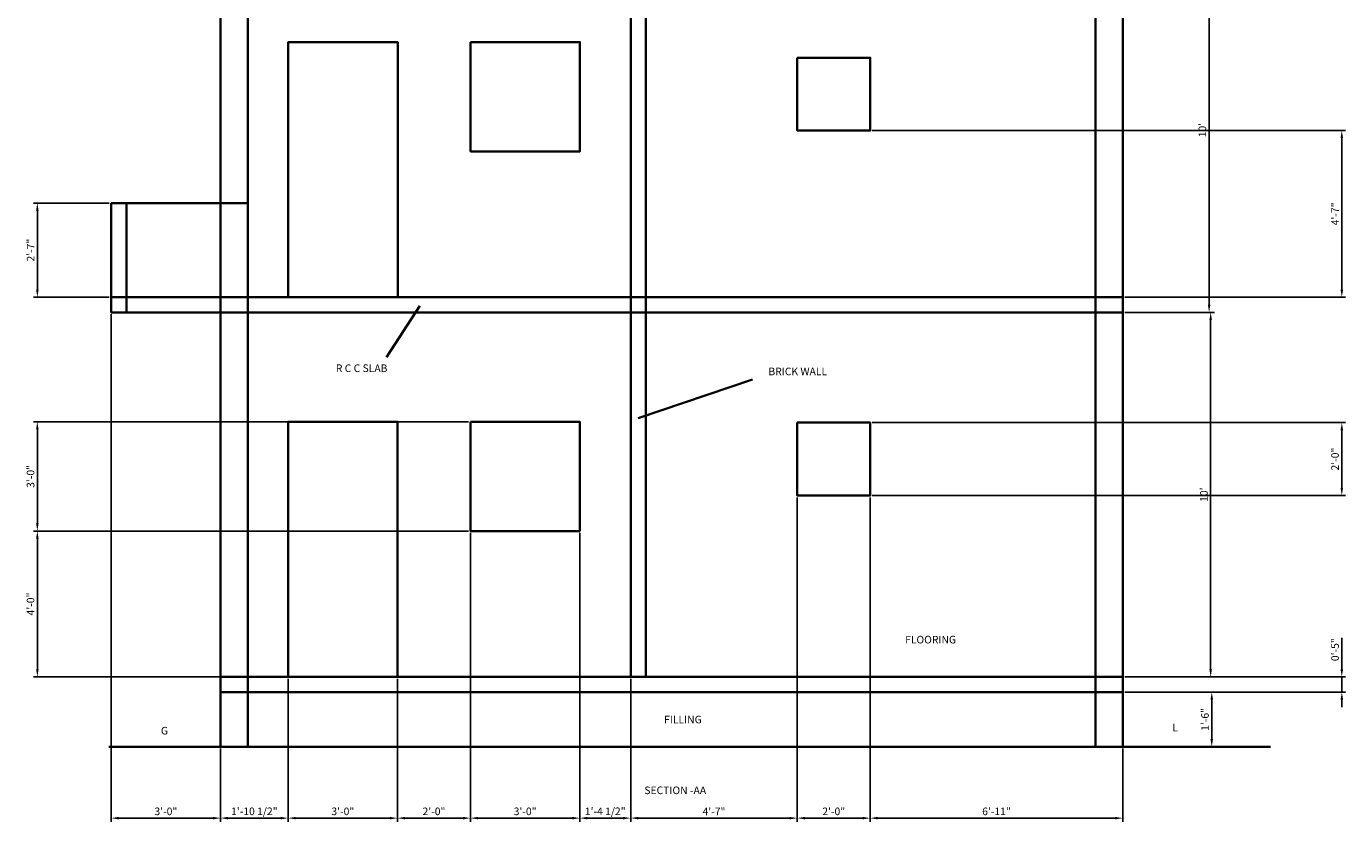
# Model space of a CAD drawing. Units: inches. Extents: x 2020 to 7901, y 1581 to 3943.
# Tile 15 of 17: x 2896 to 3331, y 2466 to 2728. Entities that reach past the tile are written whole.
import ezdxf

# ---------------------------------------------------------------- set-up
doc = ezdxf.new("R2010")
doc.units = ezdxf.units.IN
for name, color, linetype, lineweight in [('A-ANNO-DIMS', 2, 'Continuous', 18), ('A-ANNO-TEXT', 7, 'Continuous', 18), ('A-SECT', 7, 'Continuous', 35)]:
    doc.layers.add(name, color=color, linetype=linetype, lineweight=lineweight)
doc.styles.get("Standard").update_dxf_attribs({"font": 'arial.ttf'})
doc.dimstyles.new('ISO-25', dxfattribs={"dimtxt": 2.5, "dimasz": 2.5, "dimexe": 1.25, "dimexo": 0.625, "dimtad": 1, "dimdec": 1, "dimlunit": 3, "dimtxsty": 'Standard', "dimcen": 2.5, "dimadec": 0, "dimazin": 0, "dimtfac": 1, "dimtdec": 1, "dimtmove": 0, "dimatfit": 3, "dimfxl": 1, "dimarcsym": 0})

# ---------------------------------------------------------------- blocks, each defined once
blk = doc.blocks.new('*D18')
at = {"layer": 'A-ANNO-DIMS', "color": 0, "lineweight": -2, "transparency": 16777216}
for p, q in [((3272.91, 2754.21), (3286.95, 2754.21)), ((3285.7, 2751.71), (3285.7, 2636.71)), ((3257.93, 2634.21), (3286.95, 2634.21))]:
    blk.add_line(p, q, dxfattribs=at)
at = {"layer": 'A-ANNO-DIMS', "color": 0, "transparency": 16777216}
for points in [[(3285.28, 2751.71), (3286.12, 2751.71), (3285.7, 2754.21)], [(3285.28, 2636.71), (3286.12, 2636.71), (3285.7, 2634.21)]]:
    blk.add_solid(points, dxfattribs=at)
at = {"layer": 'DEFPOINTS', "color": 0, "transparency": 16777216}
for p in [(3272.28, 2754.21), (3257.31, 2634.21), (3285.7, 2634.21)]:
    blk.add_point(p, dxfattribs=at)
at = {"layer": 'A-ANNO-DIMS', "color": 0, "transparency": 16777216, "insert": (3283.8, 2694.21), "char_height": 2.5, "attachment_point": 5, "rotation": 90}
blk.add_mtext("10'", dxfattribs=at)
blk = doc.blocks.new('*D19')
at = {"layer": 'A-ANNO-DIMS', "color": 0, "lineweight": -2, "transparency": 16777216}
for p, q in [((3257.93, 2634.21), (3287.46, 2634.21)), ((3286.21, 2631.71), (3286.21, 2516.71)), ((3257.93, 2514.21), (3287.46, 2514.21))]:
    blk.add_line(p, q, dxfattribs=at)
at = {"layer": 'A-ANNO-DIMS', "color": 0, "transparency": 16777216}
for points in [[(3285.79, 2631.71), (3286.63, 2631.71), (3286.21, 2634.21)], [(3285.79, 2516.71), (3286.63, 2516.71), (3286.21, 2514.21)]]:
    blk.add_solid(points, dxfattribs=at)
at = {"layer": 'DEFPOINTS', "color": 0, "transparency": 16777216}
for p in [(3257.31, 2634.21), (3257.31, 2514.21), (3286.21, 2514.21)]:
    blk.add_point(p, dxfattribs=at)
at = {"layer": 'A-ANNO-DIMS', "color": 0, "transparency": 16777216, "insert": (3284.31, 2574.21), "char_height": 2.5, "attachment_point": 5, "rotation": 90}
blk.add_mtext("10'", dxfattribs=at)
blk = doc.blocks.new('*D20')
at = {"layer": 'A-ANNO-DIMS', "color": 0, "lineweight": -2, "transparency": 16777216}
for p, q in [((3257.93, 2509.21), (3287.82, 2509.21)), ((3286.57, 2506.71), (3286.57, 2493.71)), ((3257.93, 2491.21), (3287.82, 2491.21))]:
    blk.add_line(p, q, dxfattribs=at)
at = {"layer": 'A-ANNO-DIMS', "color": 0, "transparency": 16777216}
for points in [[(3286.15, 2506.71), (3286.99, 2506.71), (3286.57, 2509.21)], [(3286.15, 2493.71), (3286.99, 2493.71), (3286.57, 2491.21)]]:
    blk.add_solid(points, dxfattribs=at)
at = {"layer": 'DEFPOINTS', "color": 0, "transparency": 16777216}
for p in [(3257.31, 2509.21), (3257.31, 2491.21), (3286.57, 2491.21)]:
    blk.add_point(p, dxfattribs=at)
at = {"layer": 'A-ANNO-DIMS', "color": 0, "transparency": 16777216, "insert": (3284.67, 2500.21), "char_height": 2.5, "attachment_point": 5, "rotation": 90}
blk.add_mtext('1\'-6"', dxfattribs=at)
blk = doc.blocks.new('*D82')
at = {"layer": 'A-ANNO-DIMS', "color": 0, "lineweight": -2, "transparency": 16777216}
for p, q in [((2924.31, 2633.58), (2924.31, 2466.46)), ((2960.31, 2490.58), (2960.31, 2466.46)), ((2926.81, 2467.71), (2957.81, 2467.71))]:
    blk.add_line(p, q, dxfattribs=at)
at = {"layer": 'A-ANNO-DIMS', "color": 0, "transparency": 16777216}
for points in [[(2926.81, 2468.12), (2926.81, 2467.29), (2924.31, 2467.71)], [(2957.81, 2468.12), (2957.81, 2467.29), (2960.31, 2467.71)]]:
    blk.add_solid(points, dxfattribs=at)
at = {"layer": 'DEFPOINTS', "color": 0, "transparency": 16777216}
for p in [(2924.31, 2634.21), (2960.31, 2491.21), (2960.31, 2467.71)]:
    blk.add_point(p, dxfattribs=at)
at = {"layer": 'A-ANNO-DIMS', "color": 0, "transparency": 16777216, "insert": (2942.31, 2469.61), "char_height": 2.5, "attachment_point": 5}
blk.add_mtext('3\'-0"', dxfattribs=at)
blk = doc.blocks.new('*D83')
at = {"layer": 'A-ANNO-DIMS', "color": 0, "lineweight": -2, "transparency": 16777216}
for p, q in [((2982.56, 2513.58), (2982.56, 2466.46)), ((2960.31, 2490.58), (2960.31, 2466.46)), ((2962.81, 2467.71), (2980.06, 2467.71))]:
    blk.add_line(p, q, dxfattribs=at)
at = {"layer": 'A-ANNO-DIMS', "color": 0, "transparency": 16777216}
for points in [[(2962.81, 2468.12), (2962.81, 2467.29), (2960.31, 2467.71)], [(2980.06, 2468.12), (2980.06, 2467.29), (2982.56, 2467.71)]]:
    blk.add_solid(points, dxfattribs=at)
at = {"layer": 'DEFPOINTS', "color": 0, "transparency": 16777216}
for p in [(2982.56, 2514.21), (2960.31, 2491.21), (2982.56, 2467.71)]:
    blk.add_point(p, dxfattribs=at)
at = {"layer": 'A-ANNO-DIMS', "color": 0, "transparency": 16777216, "insert": (2971.43, 2469.63), "char_height": 2.5, "attachment_point": 5}
blk.add_mtext('1\'-10 1/2"', dxfattribs=at)
blk = doc.blocks.new('*D84')
at = {"layer": 'A-ANNO-DIMS', "color": 0, "lineweight": -2, "transparency": 16777216}
for p, q in [((2982.56, 2513.58), (2982.56, 2466.46)), ((3018.56, 2513.58), (3018.56, 2466.46)), ((2985.06, 2467.71), (3016.06, 2467.71))]:
    blk.add_line(p, q, dxfattribs=at)
at = {"layer": 'A-ANNO-DIMS', "color": 0, "transparency": 16777216}
for points in [[(2985.06, 2468.12), (2985.06, 2467.29), (2982.56, 2467.71)], [(3016.06, 2468.12), (3016.06, 2467.29), (3018.56, 2467.71)]]:
    blk.add_solid(points, dxfattribs=at)
at = {"layer": 'DEFPOINTS', "color": 0, "transparency": 16777216}
for p in [(2982.56, 2514.21), (3018.56, 2514.21), (3018.56, 2467.71)]:
    blk.add_point(p, dxfattribs=at)
at = {"layer": 'A-ANNO-DIMS', "color": 0, "transparency": 16777216, "insert": (3000.56, 2469.61), "char_height": 2.5, "attachment_point": 5}
blk.add_mtext('3\'-0"', dxfattribs=at)
blk = doc.blocks.new('*D85')
at = {"layer": 'A-ANNO-DIMS', "color": 0, "lineweight": -2, "transparency": 16777216}
for p, q in [((3042.56, 2561.58), (3042.56, 2466.46)), ((3018.56, 2513.58), (3018.56, 2466.46)), ((3021.06, 2467.71), (3040.06, 2467.71))]:
    blk.add_line(p, q, dxfattribs=at)
at = {"layer": 'A-ANNO-DIMS', "color": 0, "transparency": 16777216}
for points in [[(3021.06, 2468.12), (3021.06, 2467.29), (3018.56, 2467.71)], [(3040.06, 2468.12), (3040.06, 2467.29), (3042.56, 2467.71)]]:
    blk.add_solid(points, dxfattribs=at)
at = {"layer": 'DEFPOINTS', "color": 0, "transparency": 16777216}
for p in [(3042.56, 2562.21), (3018.56, 2514.21), (3042.56, 2467.71)]:
    blk.add_point(p, dxfattribs=at)
at = {"layer": 'A-ANNO-DIMS', "color": 0, "transparency": 16777216, "insert": (3030.56, 2469.61), "char_height": 2.5, "attachment_point": 5}
blk.add_mtext('2\'-0"', dxfattribs=at)
blk = doc.blocks.new('*D86')
at = {"layer": 'A-ANNO-DIMS', "color": 0, "lineweight": -2, "transparency": 16777216}
for p, q in [((3042.56, 2561.58), (3042.56, 2466.46)), ((3078.56, 2561.58), (3078.56, 2466.46)), ((3045.06, 2467.71), (3076.06, 2467.71))]:
    blk.add_line(p, q, dxfattribs=at)
at = {"layer": 'A-ANNO-DIMS', "color": 0, "transparency": 16777216}
for points in [[(3045.06, 2468.12), (3045.06, 2467.29), (3042.56, 2467.71)], [(3076.06, 2468.12), (3076.06, 2467.29), (3078.56, 2467.71)]]:
    blk.add_solid(points, dxfattribs=at)
at = {"layer": 'DEFPOINTS', "color": 0, "transparency": 16777216}
for p in [(3042.56, 2562.21), (3078.56, 2562.21), (3078.56, 2467.71)]:
    blk.add_point(p, dxfattribs=at)
at = {"layer": 'A-ANNO-DIMS', "color": 0, "transparency": 16777216, "insert": (3060.56, 2469.61), "char_height": 2.5, "attachment_point": 5}
blk.add_mtext('3\'-0"', dxfattribs=at)
blk = doc.blocks.new('*D87')
at = {"layer": 'A-ANNO-DIMS', "color": 0, "lineweight": -2, "transparency": 16777216}
for p, q in [((3078.56, 2561.58), (3078.56, 2466.46)), ((3095.31, 2513.58), (3095.31, 2466.46)), ((3081.06, 2467.71), (3092.81, 2467.71))]:
    blk.add_line(p, q, dxfattribs=at)
at = {"layer": 'A-ANNO-DIMS', "color": 0, "transparency": 16777216}
for points in [[(3081.06, 2468.12), (3081.06, 2467.29), (3078.56, 2467.71)], [(3092.81, 2468.12), (3092.81, 2467.29), (3095.31, 2467.71)]]:
    blk.add_solid(points, dxfattribs=at)
at = {"layer": 'DEFPOINTS', "color": 0, "transparency": 16777216}
for p in [(3078.56, 2562.21), (3095.31, 2514.21), (3095.31, 2467.71)]:
    blk.add_point(p, dxfattribs=at)
at = {"layer": 'A-ANNO-DIMS', "color": 0, "transparency": 16777216, "insert": (3086.93, 2469.63), "char_height": 2.5, "attachment_point": 5}
blk.add_mtext('1\'-4 1/2"', dxfattribs=at)
blk = doc.blocks.new('*D88')
at = {"layer": 'A-ANNO-DIMS', "color": 0, "lineweight": -2, "transparency": 16777216}
for p, q in [((3150.14, 2573.3), (3150.14, 2466.46)), ((3095.31, 2513.58), (3095.31, 2466.46)), ((3097.81, 2467.71), (3147.64, 2467.71))]:
    blk.add_line(p, q, dxfattribs=at)
at = {"layer": 'A-ANNO-DIMS', "color": 0, "transparency": 16777216}
for points in [[(3097.81, 2468.12), (3097.81, 2467.29), (3095.31, 2467.71)], [(3147.64, 2468.12), (3147.64, 2467.29), (3150.14, 2467.71)]]:
    blk.add_solid(points, dxfattribs=at)
at = {"layer": 'DEFPOINTS', "color": 0, "transparency": 16777216}
for p in [(3150.14, 2573.92), (3095.31, 2514.21), (3150.14, 2467.71)]:
    blk.add_point(p, dxfattribs=at)
at = {"layer": 'A-ANNO-DIMS', "color": 0, "transparency": 16777216, "insert": (3122.72, 2469.58), "char_height": 2.5, "attachment_point": 5}
blk.add_mtext('4\'-7"', dxfattribs=at)
blk = doc.blocks.new('*D89')
at = {"layer": 'A-ANNO-DIMS', "color": 0, "lineweight": -2, "transparency": 16777216}
for p, q in [((3150.14, 2573.3), (3150.14, 2466.46)), ((3174.14, 2573.3), (3174.14, 2466.46)), ((3152.64, 2467.71), (3171.64, 2467.71))]:
    blk.add_line(p, q, dxfattribs=at)
at = {"layer": 'A-ANNO-DIMS', "color": 0, "transparency": 16777216}
for points in [[(3152.64, 2468.12), (3152.64, 2467.29), (3150.14, 2467.71)], [(3171.64, 2468.12), (3171.64, 2467.29), (3174.14, 2467.71)]]:
    blk.add_solid(points, dxfattribs=at)
at = {"layer": 'DEFPOINTS', "color": 0, "transparency": 16777216}
for p in [(3150.14, 2573.92), (3174.14, 2573.92), (3174.14, 2467.71)]:
    blk.add_point(p, dxfattribs=at)
at = {"layer": 'A-ANNO-DIMS', "color": 0, "transparency": 16777216, "insert": (3162.14, 2469.61), "char_height": 2.5, "attachment_point": 5}
blk.add_mtext('2\'-0"', dxfattribs=at)
blk = doc.blocks.new('*D90')
at = {"layer": 'A-ANNO-DIMS', "color": 0, "lineweight": -2, "transparency": 16777216}
for p, q in [((3174.14, 2573.3), (3174.14, 2466.46)), ((3257.31, 2490.58), (3257.31, 2466.46)), ((3176.64, 2467.71), (3254.81, 2467.71))]:
    blk.add_line(p, q, dxfattribs=at)
at = {"layer": 'A-ANNO-DIMS', "color": 0, "transparency": 16777216}
for points in [[(3176.64, 2468.12), (3176.64, 2467.29), (3174.14, 2467.71)], [(3254.81, 2468.12), (3254.81, 2467.29), (3257.31, 2467.71)]]:
    blk.add_solid(points, dxfattribs=at)
at = {"layer": 'DEFPOINTS', "color": 0, "transparency": 16777216}
for p in [(3174.14, 2573.92), (3257.31, 2491.21), (3257.31, 2467.71)]:
    blk.add_point(p, dxfattribs=at)
at = {"layer": 'A-ANNO-DIMS', "color": 0, "transparency": 16777216, "insert": (3215.72, 2469.61), "char_height": 2.5, "attachment_point": 5}
blk.add_mtext('6\'-11"', dxfattribs=at)
blk = doc.blocks.new('*D91')
at = {"layer": 'A-ANNO-DIMS', "color": 0, "lineweight": -2, "transparency": 16777216}
for p, q in [((3041.94, 2562.21), (2898.75, 2562.21)), ((2900, 2516.71), (2900, 2559.71)), ((2981.94, 2514.21), (2898.75, 2514.21))]:
    blk.add_line(p, q, dxfattribs=at)
at = {"layer": 'A-ANNO-DIMS', "color": 0, "transparency": 16777216}
for points in [[(2899.59, 2559.71), (2900.42, 2559.71), (2900, 2562.21)], [(2899.59, 2516.71), (2900.42, 2516.71), (2900, 2514.21)]]:
    blk.add_solid(points, dxfattribs=at)
at = {"layer": 'DEFPOINTS', "color": 0, "transparency": 16777216}
for p in [(2900, 2562.21), (3042.56, 2562.21), (2982.56, 2514.21)]:
    blk.add_point(p, dxfattribs=at)
at = {"layer": 'A-ANNO-DIMS', "color": 0, "transparency": 16777216, "insert": (2898.1, 2538.21), "char_height": 2.5, "attachment_point": 5, "rotation": 90}
blk.add_mtext('4\'-0"', dxfattribs=at)
blk = doc.blocks.new('*D92')
at = {"layer": 'A-ANNO-DIMS', "color": 0, "lineweight": -2, "transparency": 16777216}
for p, q in [((3041.94, 2598.21), (2898.75, 2598.21)), ((2900, 2564.71), (2900, 2595.71)), ((3041.94, 2562.21), (2898.75, 2562.21))]:
    blk.add_line(p, q, dxfattribs=at)
at = {"layer": 'A-ANNO-DIMS', "color": 0, "transparency": 16777216}
for points in [[(2899.59, 2595.71), (2900.42, 2595.71), (2900, 2598.21)], [(2899.59, 2564.71), (2900.42, 2564.71), (2900, 2562.21)]]:
    blk.add_solid(points, dxfattribs=at)
at = {"layer": 'DEFPOINTS', "color": 0, "transparency": 16777216}
for p in [(2900, 2598.21), (3042.56, 2598.21), (3042.56, 2562.21)]:
    blk.add_point(p, dxfattribs=at)
at = {"layer": 'A-ANNO-DIMS', "color": 0, "transparency": 16777216, "insert": (2898.1, 2580.21), "char_height": 2.5, "attachment_point": 5, "rotation": 90}
blk.add_mtext('3\'-0"', dxfattribs=at)
blk = doc.blocks.new('*D93')
at = {"layer": 'A-ANNO-DIMS', "color": 0, "lineweight": -2, "transparency": 16777216}
for p, q in [((2923.68, 2670.21), (2898.75, 2670.21)), ((2900, 2641.71), (2900, 2667.71)), ((2923.68, 2639.21), (2898.75, 2639.21))]:
    blk.add_line(p, q, dxfattribs=at)
at = {"layer": 'A-ANNO-DIMS', "color": 0, "transparency": 16777216}
for points in [[(2899.59, 2667.71), (2900.42, 2667.71), (2900, 2670.21)], [(2899.59, 2641.71), (2900.42, 2641.71), (2900, 2639.21)]]:
    blk.add_solid(points, dxfattribs=at)
at = {"layer": 'DEFPOINTS', "color": 0, "transparency": 16777216}
for p in [(2900, 2670.21), (2924.31, 2670.21), (2924.31, 2639.21)]:
    blk.add_point(p, dxfattribs=at)
at = {"layer": 'A-ANNO-DIMS', "color": 0, "transparency": 16777216, "insert": (2898.12, 2654.71), "char_height": 2.5, "attachment_point": 5, "rotation": 90}
blk.add_mtext('2\'-7"', dxfattribs=at)
blk = doc.blocks.new('*D94')
at = {"layer": 'A-ANNO-DIMS', "color": 0, "lineweight": -2, "transparency": 16777216}
for p, q in [((3174.76, 2597.92), (3330.63, 2597.92)), ((3329.38, 2576.42), (3329.38, 2595.42)), ((3174.76, 2573.92), (3330.63, 2573.92))]:
    blk.add_line(p, q, dxfattribs=at)
at = {"layer": 'A-ANNO-DIMS', "color": 0, "transparency": 16777216}
for points in [[(3328.96, 2595.42), (3329.8, 2595.42), (3329.38, 2597.92)], [(3328.96, 2576.42), (3329.8, 2576.42), (3329.38, 2573.92)]]:
    blk.add_solid(points, dxfattribs=at)
at = {"layer": 'DEFPOINTS', "color": 0, "transparency": 16777216}
for p in [(3174.14, 2597.92), (3329.38, 2597.92), (3174.14, 2573.92)]:
    blk.add_point(p, dxfattribs=at)
at = {"layer": 'A-ANNO-DIMS', "color": 0, "transparency": 16777216, "insert": (3327.48, 2585.92), "char_height": 2.5, "attachment_point": 5, "rotation": 90}
blk.add_mtext('2\'-0"', dxfattribs=at)
blk = doc.blocks.new('*D160')
at = {"layer": 'A-ANNO-DIMS', "color": 0, "lineweight": -2, "transparency": 16777216}
for p, q in [((3329.38, 2516.71), (3329.38, 2527.1)), ((3257.93, 2514.21), (3330.63, 2514.21)), ((3329.38, 2509.21), (3329.38, 2514.21)), ((3257.93, 2509.21), (3330.63, 2509.21)), ((3329.38, 2506.71), (3329.38, 2504.21))]:
    blk.add_line(p, q, dxfattribs=at)
at = {"layer": 'A-ANNO-DIMS', "color": 0, "transparency": 16777216}
for points in [[(3328.96, 2516.71), (3329.8, 2516.71), (3329.38, 2514.21)], [(3328.96, 2506.71), (3329.8, 2506.71), (3329.38, 2509.21)]]:
    blk.add_solid(points, dxfattribs=at)
at = {"layer": 'DEFPOINTS', "color": 0, "transparency": 16777216}
for p in [(3257.31, 2514.21), (3329.38, 2514.21), (3257.31, 2509.21)]:
    blk.add_point(p, dxfattribs=at)
at = {"layer": 'A-ANNO-DIMS', "color": 0, "transparency": 16777216, "insert": (3327.48, 2523.16), "char_height": 2.5, "attachment_point": 5, "rotation": 90}
blk.add_mtext('0\'-5"', dxfattribs=at)
blk = doc.blocks.new('*D165')
at = {"layer": 'A-ANNO-DIMS', "color": 0, "lineweight": -2, "transparency": 16777216}
for p, q in [((3174.76, 2694.07), (3330.63, 2694.07)), ((3329.38, 2691.57), (3329.38, 2641.71)), ((3257.93, 2639.21), (3330.63, 2639.21))]:
    blk.add_line(p, q, dxfattribs=at)
at = {"layer": 'A-ANNO-DIMS', "color": 0, "transparency": 16777216}
for points in [[(3328.96, 2691.57), (3329.8, 2691.57), (3329.38, 2694.07)], [(3328.96, 2641.71), (3329.8, 2641.71), (3329.38, 2639.21)]]:
    blk.add_solid(points, dxfattribs=at)
at = {"layer": 'DEFPOINTS', "color": 0, "transparency": 16777216}
for p in [(3174.14, 2694.07), (3257.31, 2639.21), (3329.38, 2639.21)]:
    blk.add_point(p, dxfattribs=at)
at = {"layer": 'A-ANNO-DIMS', "color": 0, "transparency": 16777216, "insert": (3327.5, 2666.64), "char_height": 2.5, "attachment_point": 5, "rotation": 90}
blk.add_mtext('4\'-7"', dxfattribs=at)

msp = doc.modelspace()

# ---------------------------------------------------------------- linework, layer by layer
at = {"layer": 'A-SECT'}
for p, q in [((3257.31, 2491.21), (3257.31, 2915.21)), ((3248.31, 2491.21), (3248.31, 2879.21)), ((2960.31, 2491.21), (2960.31, 2874.21)), ((2969.31, 2491.21), (2969.31, 2874.21)), ((3095.31, 2514.21), (3095.31, 2874.21)), ((3100.31, 2514.21), (3100.31, 2874.21)), ((2924.31, 2634.21), (2924.31, 2670.21)), ((2924.31, 2670.21), (2969.31, 2670.21)), ((2929.31, 2634.21), (2929.31, 2670.21)), ((2960.31, 2639.21), (2924.31, 2639.21)), ((3257.31, 2639.21), (2960.31, 2639.21)), ((3025.93, 2636.34), (3014.93, 2619.49)), ((2960.31, 2634.21), (2924.31, 2634.21)), ((3257.31, 2634.21), (2960.31, 2634.21)), ((3097.74, 2599.39), (3135.41, 2612.16)), ((3257.31, 2514.21), (2960.31, 2514.21)), ((3257.31, 2509.21), (2960.31, 2509.21)), ((2960.31, 2491.21), (2923.5, 2491.21)), ((3257.31, 2491.21), (2960.31, 2491.21)), ((3257.31, 2491.21), (3305.88, 2491.21))]:
    msp.add_line(p, q, dxfattribs=at)
for points in [[(2982.61, 2639.21), (3018.61, 2639.21), (3018.61, 2723.21), (2982.61, 2723.21)], [(3042.61, 2723.21), (3078.61, 2723.21), (3078.61, 2687.21), (3042.61, 2687.21)], [(3150.14, 2718.07), (3174.14, 2718.07), (3174.14, 2694.07), (3150.14, 2694.07)], [(2982.56, 2514.21), (3018.56, 2514.21), (3018.56, 2598.21), (2982.56, 2598.21)], [(3042.56, 2598.21), (3078.56, 2598.21), (3078.56, 2562.21), (3042.56, 2562.21)], [(3150.14, 2597.92), (3174.14, 2597.92), (3174.14, 2573.92), (3150.14, 2573.92)]]:
    msp.add_lwpolyline(points, close=True, dxfattribs=at)

# ---------------------------------------------------------------- texts
at = {"layer": 'A-ANNO-TEXT', "char_height": 2.5, "attachment_point": 1}
for s, width, insert in [('R C C SLAB', 71.4175, (2998.25, 2617.08)), ('BRICK WALL', 38.9877, (3140.63, 2616.01)), ('FLOORING', 51.5386, (3185.64, 2527.72)), ('FILLING', 48.9773, (3106.3, 2501.41)), ('G', 17.1043, (2940.67, 2497.74)), ('L', 14.1332, (3273.59, 2498.76)), ('SECTION -AA', 154.0816, (3099.79, 2478.11))]:
    msp.add_mtext_dynamic_manual_height_columns(s, width=width, gutter_width=12.5, heights=[0], dxfattribs=dict(at, insert=insert))

# ---------------------------------------------------------------- dimensions: what is measured, and where the dimension line sits
at = {"layer": 'A-ANNO-DIMS'}
for base, p1, p2, override, picture, middle in [((3285.7, 2634.21), (3272.28, 2754.21), (3257.31, 2634.21), {"dimclrd": 0, "dimclre": 0, "dimclrt": 0}, '*D18', (3283.8, 2694.21)), ((3329.38, 2639.21), (3174.14, 2694.07), (3257.31, 2639.21), {"dimdec": 1, "dimlfac": 1, "dimrnd": 0, "dimzin": 1, "dimdsep": 46, "dimlunit": 4, "dimfrac": 2}, '*D165', (3327.5, 2666.64)), ((2900, 2670.21), (2924.31, 2639.21), (2924.31, 2670.21), {"dimdec": 1, "dimlfac": 1, "dimrnd": 0, "dimzin": 1, "dimdsep": 46, "dimlunit": 4, "dimfrac": 2}, '*D93', (2898.12, 2654.71)), ((3286.21, 2514.21), (3257.31, 2634.21), (3257.31, 2514.21), {"dimclrd": 0, "dimclre": 0, "dimclrt": 0}, '*D19', (3284.31, 2574.21)), ((2900, 2598.21), (3042.56, 2562.21), (3042.56, 2598.21), {"dimdec": 1, "dimlfac": 1, "dimrnd": 0, "dimzin": 1, "dimdsep": 46, "dimlunit": 4, "dimfrac": 2}, '*D92', (2898.1, 2580.21)), ((3329.38, 2597.92), (3174.14, 2573.92), (3174.14, 2597.92), {"dimdec": 1, "dimlfac": 1, "dimrnd": 0, "dimzin": 1, "dimdsep": 46, "dimlunit": 4, "dimfrac": 2}, '*D94', (3327.48, 2585.92)), ((2900, 2562.21), (2982.56, 2514.21), (3042.56, 2562.21), {"dimdec": 1, "dimlfac": 1, "dimrnd": 0, "dimzin": 1, "dimdsep": 46, "dimlunit": 4, "dimfrac": 2}, '*D91', (2898.1, 2538.21)), ((3329.38, 2514.21), (3257.31, 2509.21), (3257.31, 2514.21), {"dimdec": 1, "dimlfac": 1, "dimrnd": 0, "dimzin": 1, "dimdsep": 46, "dimlunit": 4, "dimfrac": 2}, '*D160', (3327.48, 2523.16)), ((3286.57, 2491.21), (3257.31, 2509.21), (3257.31, 2491.21), {"dimclrd": 0, "dimclre": 0, "dimclrt": 0}, '*D20', (3284.67, 2500.21))]:
    dim = msp.add_linear_dim(base=base, p1=p1, p2=p2, angle=90, dimstyle='ISO-25', override=override, dxfattribs=at)
    dim.commit()
    dim.dimension.update_dxf_attribs({"geometry": picture, "text_midpoint": middle})
for base, p1, p2, picture, middle in [((2960.31, 2467.71), (2924.31, 2634.21), (2960.31, 2491.21), '*D82', (2942.31, 2469.61)), ((3150.14, 2467.71), (3095.31, 2514.21), (3150.14, 2573.92), '*D88', (3122.72, 2469.58)), ((3174.14, 2467.71), (3150.14, 2573.92), (3174.14, 2573.92), '*D89', (3162.14, 2469.61)), ((3257.31, 2467.71), (3174.14, 2573.92), (3257.31, 2491.21), '*D90', (3215.72, 2469.61)), ((3042.56, 2467.71), (3018.56, 2514.21), (3042.56, 2562.21), '*D85', (3030.56, 2469.61)), ((3078.56, 2467.71), (3042.56, 2562.21), (3078.56, 2562.21), '*D86', (3060.56, 2469.61)), ((3095.3056, 2467.7078), (3078.5622, 2562.2078), (3095.3056, 2514.2078), '*D87', (3086.9339, 2469.6254)), ((2982.5622, 2467.7078), (2960.3056, 2491.2078), (2982.5622, 2514.2078), '*D83', (2971.4339, 2469.6254)), ((3018.56, 2467.71), (2982.56, 2514.21), (3018.56, 2514.21), '*D84', (3000.56, 2469.61))]:
    dim = msp.add_linear_dim(base=base, p1=p1, p2=p2, dimstyle='ISO-25', override={"dimdec": 1, "dimlfac": 1, "dimrnd": 0, "dimzin": 1, "dimdsep": 46, "dimlunit": 4, "dimfrac": 2}, dxfattribs=at)
    dim.commit()
    dim.dimension.update_dxf_attribs({"geometry": picture, "text_midpoint": middle})

doc.saveas('drawing.dxf')
